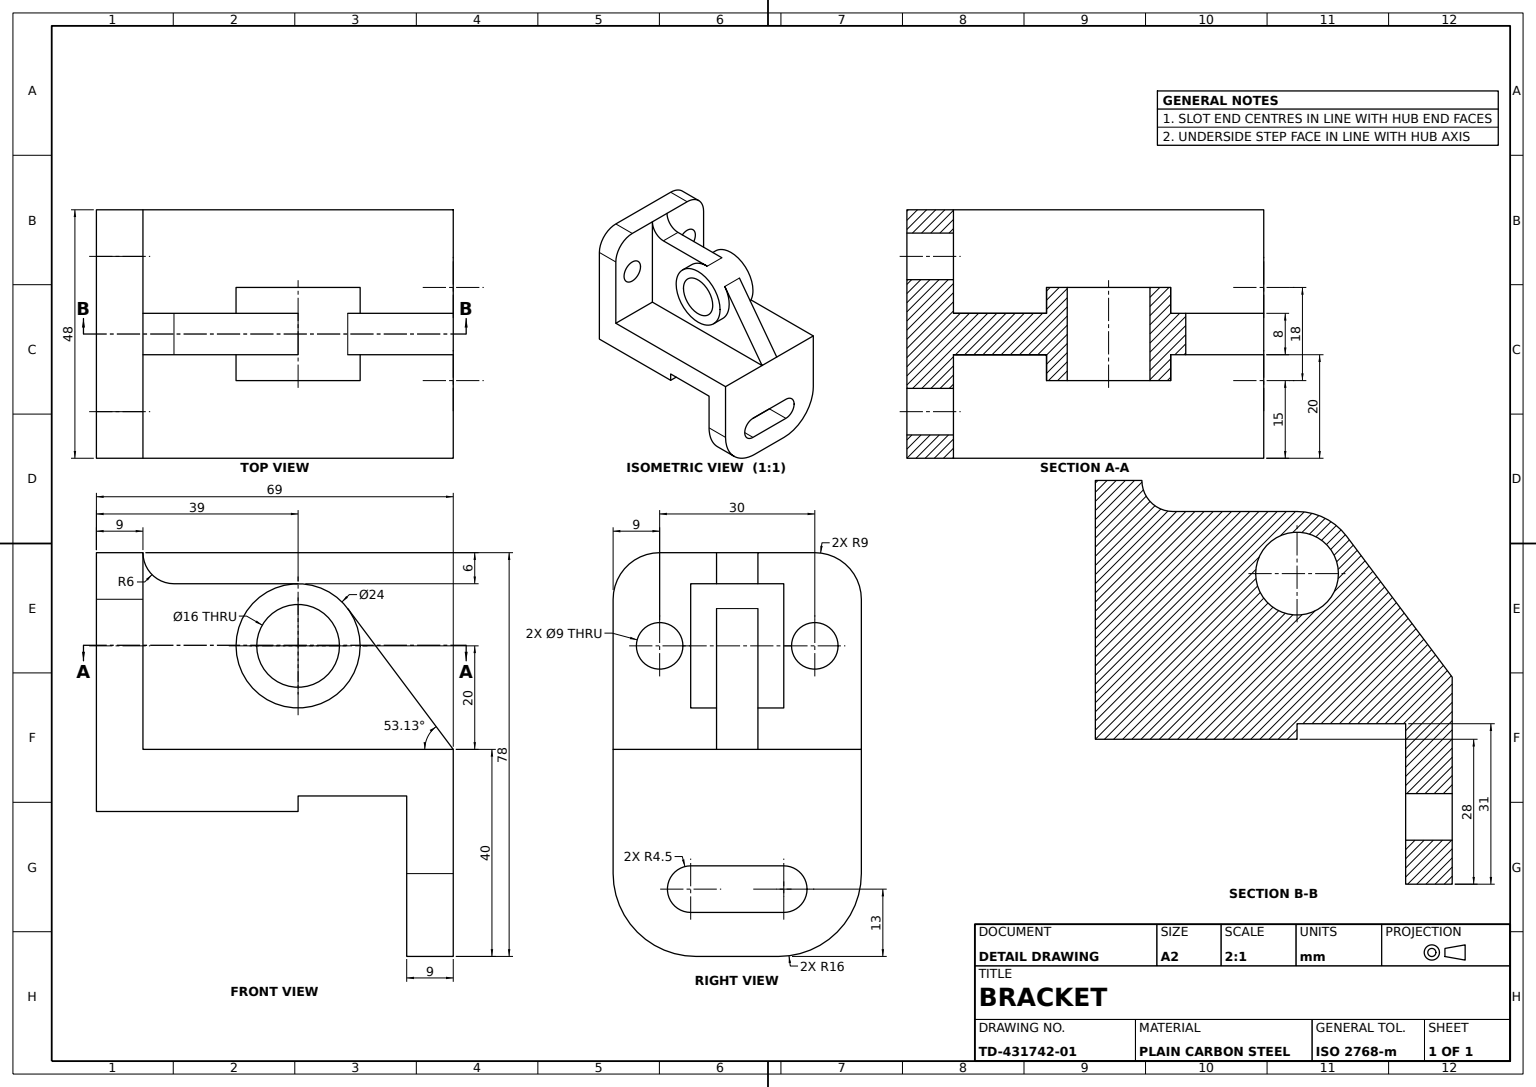
from build123d import *

# Parameters (mm, degrees)
L_BRACKET_BASE_DEPTH                      = 48
BASE_CORNER_ROUNDS_R16_R                  = 16
SLOT_CUT_DEPTH                            = 48
BACK_PLATE_SKETCH_W                       = 48
BACK_PLATE_SKETCH_H                       = 38
BACK_PLATE_SKETCH_R                       = 4.5
BACK_PLATE_WITH_MOUNTING_HOLES_2X_9_DEPTH = 9
BEARING_HUB_SKETCH_R                      = 12
BEARING_HUB_SKETCH_R_2                    = 8
BEARING_HUB_DEPTH                         = 9
SUPPORT_RIB_DEPTH                         = 4
BEARING_BORE_SKETCH_R                     = 8
BEARING_BORE_16_DEPTH                     = 90.693923986
BACK_PLATE_CORNER_ROUNDS_R9_R             = 9


with BuildPart() as part:
    # L Bracket Profile Sketch → L Bracket Base (new body)
    with BuildSketch(Plane.XY):
        Polygon((0, 0), (39, 0), (39, 3), (60, 3), (60, 0), (60, -28), (69, -28), (69, 12), (0, 12), align=None)
    extrude(amount=-L_BRACKET_BASE_DEPTH)

    # Base Corner Rounds R16
    base_corner_rounds_r16_edges = [part.edges().sort_by_distance(p)[0] for p in [
        (64.5, -28, 0),
        (64.5, -28, -48),
    ]]
    fillet(base_corner_rounds_r16_edges, radius=BASE_CORNER_ROUNDS_R16_R)

    # Slot Sketch → Slot Cut (cut)
    with BuildSketch(Plane(origin=(69, 0, 0), x_dir=(0, 0, -1), z_dir=(1, 0, 0))):
        with BuildLine():
            Line((15, -10.5), (33, -10.5))
            ThreePointArc((33, -10.5), (37.5, -15), (33, -19.5))
            Line((33, -19.5), (15, -19.5))
            ThreePointArc((15, -19.5), (10.5, -15), (15, -10.5))
        make_face()
    extrude(amount=-SLOT_CUT_DEPTH, mode=Mode.SUBTRACT)

    # Back Plate Sketch → Back Plate with Mounting Holes 2xØ9 (add)
    with BuildSketch(Plane.ZY):
        with Locations((-24, 31)):
            Rectangle(BACK_PLATE_SKETCH_W, BACK_PLATE_SKETCH_H)
        with Locations((-39, 32)):
            Circle(BACK_PLATE_SKETCH_R, mode=Mode.SUBTRACT)
        with Locations((-9, 32)):
            Circle(BACK_PLATE_SKETCH_R, mode=Mode.SUBTRACT)
    extrude(amount=-BACK_PLATE_WITH_MOUNTING_HOLES_2X_9_DEPTH)



with BuildPart() as body_2:
    # Bearing Hub Sketch → Bearing Hub (new, symmetric)
    with BuildSketch(Plane.XY.offset(-24)):
        with Locations((39, 32)):
            Circle(BEARING_HUB_SKETCH_R)
        with Locations((39, 32)):
            Circle(BEARING_HUB_SKETCH_R_2, mode=Mode.SUBTRACT)
    extrude(amount=BEARING_HUB_DEPTH, both=True)


with BuildPart() as part_1:
    add(part.part)

    add(body_2.part)  # Support Rib merges body 2
    # Support Rib Sketch → Support Rib (add, symmetric)
    with BuildSketch(Plane.XY.offset(-24)):
        with BuildLine():
            Line((69, 12), (48.6, 39.2))
            ThreePointArc((48.6, 39.2), (44.276884864, 42.553769728), (39, 44))
            Line((39, 44), (15, 44))
            ThreePointArc((15, 44), (10.757359313, 45.757359313), (9, 50))
            Line((9, 50), (9, 12))
            Line((9, 12), (69, 12))
        make_face()
    extrude(amount=SUPPORT_RIB_DEPTH, both=True)

    # Bearing Bore Sketch → Bearing Bore Ø16 (cut, through all)
    with BuildSketch(Plane.XY.offset(-20)):
        with Locations((39, 32)):
            Circle(BEARING_BORE_SKETCH_R)
    extrude(amount=-BEARING_BORE_16_DEPTH, mode=Mode.SUBTRACT)

    # Back Plate Corner Rounds R9
    back_plate_corner_rounds_r9_edges = [part_1.edges().sort_by_distance(p)[0] for p in [
        (4.5, 50, -48),
        (4.5, 50, 0),
    ]]
    fillet(back_plate_corner_rounds_r9_edges, radius=BACK_PLATE_CORNER_ROUNDS_R9_R)


solid = part_1.part
